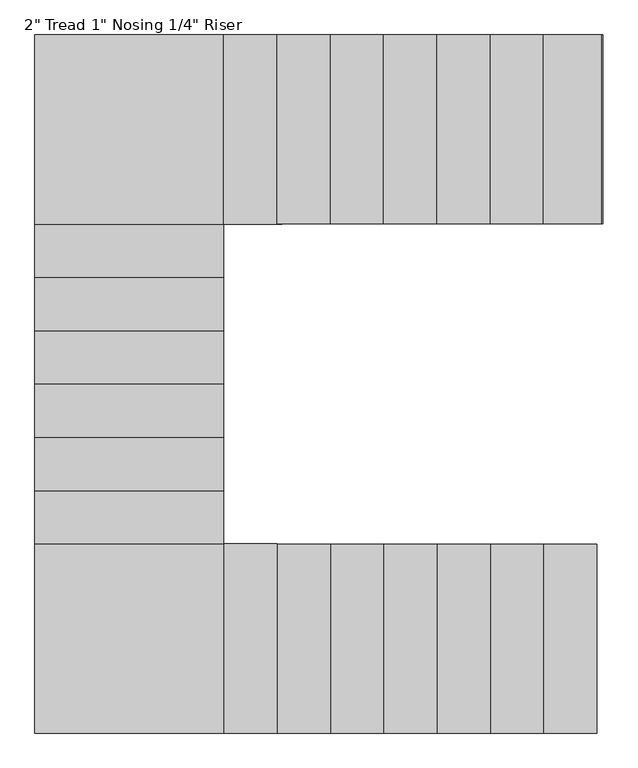
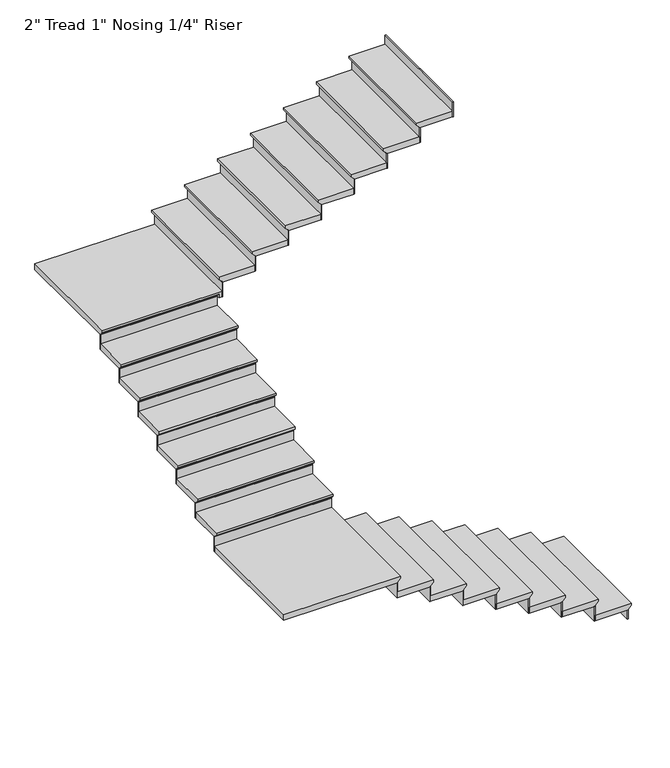
"""IFC4 building model written with IfcOpenShell, lengths in millimetres: stair flight geometry."""

from ifc_helpers import new_model, si_unit, origin, place, context, project, spatial, faceted_brep, source, transform, mapped, element, save


def stair_flight_8adf14a6(model_context):
    return source(origin(), model_context, "Body", "Brep", [
        faceted_brep([(-19769.8789184, -127.8399287, 6361.8717391), (-19769.8789184, -127.8399287, 6380.9217391), (-19769.8789184, -1118.4399287, 6380.9217391), (-19769.8789184, -1118.4399287, 6361.8717391), (-19795.2789184, -127.8399287, 6336.4717391), (-19795.2789184, -1118.4399287, 6336.4717391), (-20074.6789184, -127.8399287, 6380.9217391), (-20074.6789184, -1118.4399287, 6380.9217391), (-19795.2789184, -1118.4399287, 6330.1217391), (-20074.6789184, -1118.4399287, 6330.1217391), (-20074.6789184, -127.8399287, 6330.1217391), (-19795.2789184, -127.8399287, 6330.1217391)], [[[0, 1, 2, 3]], [[4, 0, 3, 5]], [[2, 1, 6, 7]], [[8, 9, 10, 11]], [[2, 7, 9, 8, 5, 3]], [[8, 11, 4, 5]], [[6, 1, 0, 4, 11, 10]], [[7, 6, 10, 9]]]),
        faceted_brep([(-19795.2789184, -127.8399287, 6330.1217391), (-19795.2789184, -127.8399287, 6248.4), (-19801.6289184, -127.8399287, 6248.4), (-19801.6289184, -127.8399287, 6330.1217391), (-19795.2789184, -1118.4399287, 6330.1217391), (-19801.6289184, -1118.4399287, 6330.1217391), (-19801.6289184, -1118.4399287, 6248.4), (-19795.2789184, -1118.4399287, 6248.4)], [[[0, 1, 2, 3]], [[4, 5, 6, 7]], [[1, 0, 4, 7]], [[2, 1, 7, 6]], [[3, 2, 6, 5]], [[0, 3, 5, 4]]]),
        faceted_brep([(-20074.6789184, -127.8399287, 6462.6434783), (-20074.6789184, -127.8399287, 6330.1217391), (-20081.0289184, -127.8399287, 6330.1217391), (-20081.0289184, -127.8399287, 6462.6434783), (-20074.6789184, -1118.4399287, 6462.6434783), (-20081.0289184, -1118.4399287, 6462.6434783), (-20081.0289184, -1118.4399287, 6330.1217391), (-20074.6789184, -1118.4399287, 6330.1217391)], [[[0, 1, 2, 3]], [[4, 5, 6, 7]], [[1, 0, 4, 7]], [[2, 1, 7, 6]], [[3, 2, 6, 5]], [[0, 3, 5, 4]]]),
        faceted_brep([(-20049.2789184, -1118.4399287, 6513.4434783), (-20049.2789184, -127.8399287, 6513.4434783), (-20354.0789184, -127.8399287, 6513.4434783), (-20354.0789184, -1118.4399287, 6513.4434783), (-20074.6789184, -1118.4399287, 6462.6434783), (-20354.0789184, -1118.4399287, 6462.6434783), (-20354.0789184, -127.8399287, 6462.6434783), (-20074.6789184, -127.8399287, 6462.6434783), (-20074.6789184, -1118.4399287, 6468.9934783), (-20049.2789184, -1118.4399287, 6494.3934783), (-20074.6789184, -127.8399287, 6468.9934783), (-20049.2789184, -127.8399287, 6494.3934783)], [[[0, 1, 2, 3]], [[4, 5, 6, 7]], [[0, 3, 5, 4, 8, 9]], [[4, 7, 10, 8]], [[2, 1, 11, 10, 7, 6]], [[3, 2, 6, 5]], [[11, 1, 0, 9]], [[10, 11, 9, 8]]]),
        faceted_brep([(-20354.0789184, -127.8399287, 6595.1652174), (-20354.0789184, -127.8399287, 6462.6434783), (-20360.4289184, -127.8399287, 6462.6434783), (-20360.4289184, -127.8399287, 6595.1652174), (-20354.0789184, -1118.4399287, 6595.1652174), (-20360.4289184, -1118.4399287, 6595.1652174), (-20360.4289184, -1118.4399287, 6462.6434783), (-20354.0789184, -1118.4399287, 6462.6434783)], [[[0, 1, 2, 3]], [[4, 5, 6, 7]], [[1, 0, 4, 7]], [[2, 1, 7, 6]], [[3, 2, 6, 5]], [[0, 3, 5, 4]]]),
        faceted_brep([(-20328.6789184, -1118.4399287, 6645.9652174), (-20328.6789184, -127.8399287, 6645.9652174), (-20633.4789184, -127.8399287, 6645.9652174), (-20633.4789184, -1118.4399287, 6645.9652174), (-20354.0789184, -1118.4399287, 6595.1652174), (-20633.4789184, -1118.4399287, 6595.1652174), (-20633.4789184, -127.8399287, 6595.1652174), (-20354.0789184, -127.8399287, 6595.1652174), (-20354.0789184, -1118.4399287, 6601.5152174), (-20328.6789184, -1118.4399287, 6626.9152174), (-20354.0789184, -127.8399287, 6601.5152174), (-20328.6789184, -127.8399287, 6626.9152174)], [[[0, 1, 2, 3]], [[4, 5, 6, 7]], [[0, 3, 5, 4, 8, 9]], [[4, 7, 10, 8]], [[2, 1, 11, 10, 7, 6]], [[3, 2, 6, 5]], [[11, 1, 0, 9]], [[10, 11, 9, 8]]]),
        faceted_brep([(-20633.4789184, -127.8399287, 6727.6869565), (-20633.4789184, -127.8399287, 6595.1652174), (-20639.8289184, -127.8399287, 6595.1652174), (-20639.8289184, -127.8399287, 6727.6869565), (-20633.4789184, -1118.4399287, 6727.6869565), (-20639.8289184, -1118.4399287, 6727.6869565), (-20639.8289184, -1118.4399287, 6595.1652174), (-20633.4789184, -1118.4399287, 6595.1652174)], [[[0, 1, 2, 3]], [[4, 5, 6, 7]], [[1, 0, 4, 7]], [[2, 1, 7, 6]], [[3, 2, 6, 5]], [[0, 3, 5, 4]]]),
        faceted_brep([(-20608.0789184, -1118.4399287, 6778.4869565), (-20608.0789184, -127.8399287, 6778.4869565), (-20912.8789184, -127.8399287, 6778.4869565), (-20912.8789184, -1118.4399287, 6778.4869565), (-20633.4789184, -1118.4399287, 6727.6869565), (-20912.8789184, -1118.4399287, 6727.6869565), (-20912.8789184, -127.8399287, 6727.6869565), (-20633.4789184, -127.8399287, 6727.6869565), (-20633.4789184, -1118.4399287, 6734.0369565), (-20608.0789184, -1118.4399287, 6759.4369565), (-20633.4789184, -127.8399287, 6734.0369565), (-20608.0789184, -127.8399287, 6759.4369565)], [[[0, 1, 2, 3]], [[4, 5, 6, 7]], [[0, 3, 5, 4, 8, 9]], [[4, 7, 10, 8]], [[2, 1, 11, 10, 7, 6]], [[3, 2, 6, 5]], [[11, 1, 0, 9]], [[10, 11, 9, 8]]]),
        faceted_brep([(-20912.8789184, -127.8399287, 6860.2086957), (-20912.8789184, -127.8399287, 6727.6869565), (-20919.2289184, -127.8399287, 6727.6869565), (-20919.2289184, -127.8399287, 6860.2086957), (-20912.8789184, -1118.4399287, 6860.2086957), (-20919.2289184, -1118.4399287, 6860.2086957), (-20919.2289184, -1118.4399287, 6727.6869565), (-20912.8789184, -1118.4399287, 6727.6869565)], [[[0, 1, 2, 3]], [[4, 5, 6, 7]], [[1, 0, 4, 7]], [[2, 1, 7, 6]], [[3, 2, 6, 5]], [[0, 3, 5, 4]]]),
        faceted_brep([(-20887.4789184, -1118.4399287, 6911.0086957), (-20887.4789184, -127.8399287, 6911.0086957), (-21192.2789184, -127.8399287, 6911.0086957), (-21192.2789184, -1118.4399287, 6911.0086957), (-20912.8789184, -1118.4399287, 6860.2086957), (-21192.2789184, -1118.4399287, 6860.2086957), (-21192.2789184, -127.8399287, 6860.2086957), (-20912.8789184, -127.8399287, 6860.2086957), (-20912.8789184, -1118.4399287, 6866.5586957), (-20887.4789184, -1118.4399287, 6891.9586957), (-20912.8789184, -127.8399287, 6866.5586957), (-20887.4789184, -127.8399287, 6891.9586957)], [[[0, 1, 2, 3]], [[4, 5, 6, 7]], [[0, 3, 5, 4, 8, 9]], [[4, 7, 10, 8]], [[2, 1, 11, 10, 7, 6]], [[3, 2, 6, 5]], [[11, 1, 0, 9]], [[10, 11, 9, 8]]]),
        faceted_brep([(-21192.2789184, -127.8399287, 6992.7304348), (-21192.2789184, -127.8399287, 6860.2086957), (-21198.6289184, -127.8399287, 6860.2086957), (-21198.6289184, -127.8399287, 6992.7304348), (-21192.2789184, -1118.4399287, 6992.7304348), (-21198.6289184, -1118.4399287, 6992.7304348), (-21198.6289184, -1118.4399287, 6860.2086957), (-21192.2789184, -1118.4399287, 6860.2086957)], [[[0, 1, 2, 3]], [[4, 5, 6, 7]], [[1, 0, 4, 7]], [[2, 1, 7, 6]], [[3, 2, 6, 5]], [[0, 3, 5, 4]]]),
        faceted_brep([(-21166.8789184, -1118.4399287, 7043.5304348), (-21166.8789184, -127.8399287, 7043.5304348), (-21471.6789184, -127.8399287, 7043.5304348), (-21471.6789184, -1118.4399287, 7043.5304348), (-21192.2789184, -1118.4399287, 6992.7304348), (-21471.6789184, -1118.4399287, 6992.7304348), (-21471.6789184, -127.8399287, 6992.7304348), (-21192.2789184, -127.8399287, 6992.7304348), (-21192.2789184, -1118.4399287, 6999.0804348), (-21166.8789184, -1118.4399287, 7024.4804348), (-21192.2789184, -127.8399287, 6999.0804348), (-21166.8789184, -127.8399287, 7024.4804348)], [[[0, 1, 2, 3]], [[4, 5, 6, 7]], [[0, 3, 5, 4, 8, 9]], [[4, 7, 10, 8]], [[2, 1, 11, 10, 7, 6]], [[3, 2, 6, 5]], [[11, 1, 0, 9]], [[10, 11, 9, 8]]]),
        faceted_brep([(-21471.6789184, -127.8399287, 7125.2521739), (-21471.6789184, -127.8399287, 6992.7304348), (-21478.0289184, -127.8399287, 6992.7304348), (-21478.0289184, -127.8399287, 7125.2521739), (-21471.6789184, -1118.4399287, 7125.2521739), (-21478.0289184, -1118.4399287, 7125.2521739), (-21478.0289184, -1118.4399287, 6992.7304348), (-21471.6789184, -1118.4399287, 6992.7304348)], [[[0, 1, 2, 3]], [[4, 5, 6, 7]], [[1, 0, 4, 7]], [[2, 1, 7, 6]], [[3, 2, 6, 5]], [[0, 3, 5, 4]]]),
        faceted_brep([(-21446.2789184, -1118.4399287, 7176.0521739), (-21446.2789184, -127.8399287, 7176.0521739), (-21751.0789184, -127.8399287, 7176.0521739), (-21751.0789184, -1118.4399287, 7176.0521739), (-21471.6789184, -1118.4399287, 7125.2521739), (-21751.0789184, -1118.4399287, 7125.2521739), (-21751.0789184, -127.8399287, 7125.2521739), (-21471.6789184, -127.8399287, 7125.2521739), (-21471.6789184, -1118.4399287, 7131.6021739), (-21446.2789184, -1118.4399287, 7157.0021739), (-21471.6789184, -127.8399287, 7131.6021739), (-21446.2789184, -127.8399287, 7157.0021739)], [[[0, 1, 2, 3]], [[4, 5, 6, 7]], [[0, 3, 5, 4, 8, 9]], [[4, 7, 10, 8]], [[2, 1, 11, 10, 7, 6]], [[3, 2, 6, 5]], [[11, 1, 0, 9]], [[10, 11, 9, 8]]]),
        faceted_brep([(-21751.0789184, -127.8399287, 7257.773913), (-21751.0789184, -127.8399287, 7125.2521739), (-21757.4289184, -127.8399287, 7125.2521739), (-21757.4289184, -127.8399287, 7257.773913), (-21751.0789184, -1118.4399287, 7257.773913), (-21757.4289184, -1118.4399287, 7257.773913), (-21757.4289184, -1118.4399287, 7125.2521739), (-21751.0789184, -1118.4399287, 7125.2521739)], [[[0, 1, 2, 3]], [[4, 5, 6, 7]], [[1, 0, 4, 7]], [[2, 1, 7, 6]], [[3, 2, 6, 5]], [[0, 3, 5, 4]]]),
        faceted_brep([(-22716.2789184, -102.4399287, 7308.573913), (-22716.2789184, -1118.4399287, 7308.573913), (-21725.6789184, -1118.4399287, 7308.573913), (-21725.6789184, -102.4399287, 7308.573913), (-22716.2789184, -1118.4399287, 7257.773913), (-22716.2789184, -102.4399287, 7257.773913), (-21725.6789184, -102.4399287, 7257.773913), (-21725.6789184, -127.8399287, 7257.773913), (-21751.0789184, -127.8399287, 7257.773913), (-21751.0789184, -1118.4399287, 7257.773913), (-21751.0789184, -127.8399287, 7264.123913), (-21751.0789184, -1118.4399287, 7264.123913), (-21725.6789184, -1118.4399287, 7289.523913), (-21725.6789184, -127.8399287, 7289.523913)], [[[0, 1, 2, 3]], [[4, 5, 6, 7, 8, 9]], [[1, 0, 5, 4]], [[9, 8, 10, 11]], [[3, 2, 12, 13, 7, 6]], [[0, 3, 6, 5]], [[12, 11, 10, 13]], [[2, 1, 4, 9, 11, 12]], [[8, 7, 13, 10]]]),
        faceted_brep([(-21725.6789184, -102.4399287, 7390.2956522), (-21725.6789184, -102.4399287, 7257.773913), (-21725.6789184, -96.0899287, 7257.773913), (-21725.6789184, -96.0899287, 7390.2956522), (-22716.2789184, -102.4399287, 7390.2956522), (-22716.2789184, -96.0899287, 7390.2956522), (-22716.2789184, -96.0899287, 7257.773913), (-22716.2789184, -102.4399287, 7257.773913)], [[[0, 1, 2, 3]], [[4, 5, 6, 7]], [[1, 0, 4, 7]], [[2, 1, 7, 6]], [[3, 2, 6, 5]], [[0, 3, 5, 4]]]),
        faceted_brep([(-22716.2789184, -127.8399287, 7441.0956522), (-21725.6789184, -127.8399287, 7441.0956522), (-21725.6789184, 176.9600713, 7441.0956522), (-22716.2789184, 176.9600713, 7441.0956522), (-22716.2789184, -102.4399287, 7390.2956522), (-22716.2789184, 176.9600713, 7390.2956522), (-21725.6789184, 176.9600713, 7390.2956522), (-21725.6789184, -102.4399287, 7390.2956522), (-22716.2789184, -102.4399287, 7396.6456522), (-22716.2789184, -127.8399287, 7422.0456522), (-21725.6789184, -102.4399287, 7396.6456522), (-21725.6789184, -127.8399287, 7422.0456522)], [[[0, 1, 2, 3]], [[4, 5, 6, 7]], [[0, 3, 5, 4, 8, 9]], [[4, 7, 10, 8]], [[2, 1, 11, 10, 7, 6]], [[3, 2, 6, 5]], [[11, 1, 0, 9]], [[10, 11, 9, 8]]]),
        faceted_brep([(-21725.6789184, 176.9600713, 7522.8173913), (-21725.6789184, 176.9600713, 7390.2956522), (-21725.6789184, 183.3100713, 7390.2956522), (-21725.6789184, 183.3100713, 7522.8173913), (-22716.2789184, 176.9600713, 7522.8173913), (-22716.2789184, 183.3100713, 7522.8173913), (-22716.2789184, 183.3100713, 7390.2956522), (-22716.2789184, 176.9600713, 7390.2956522)], [[[0, 1, 2, 3]], [[4, 5, 6, 7]], [[1, 0, 4, 7]], [[2, 1, 7, 6]], [[3, 2, 6, 5]], [[0, 3, 5, 4]]]),
        faceted_brep([(-22716.2789184, 151.5600713, 7573.6173913), (-21725.6789184, 151.5600713, 7573.6173913), (-21725.6789184, 456.3600713, 7573.6173913), (-22716.2789184, 456.3600713, 7573.6173913), (-22716.2789184, 176.9600713, 7522.8173913), (-22716.2789184, 456.3600713, 7522.8173913), (-21725.6789184, 456.3600713, 7522.8173913), (-21725.6789184, 176.9600713, 7522.8173913), (-22716.2789184, 176.9600713, 7529.1673913), (-22716.2789184, 151.5600713, 7554.5673913), (-21725.6789184, 176.9600713, 7529.1673913), (-21725.6789184, 151.5600713, 7554.5673913)], [[[0, 1, 2, 3]], [[4, 5, 6, 7]], [[0, 3, 5, 4, 8, 9]], [[4, 7, 10, 8]], [[2, 1, 11, 10, 7, 6]], [[3, 2, 6, 5]], [[11, 1, 0, 9]], [[10, 11, 9, 8]]]),
        faceted_brep([(-21725.6789184, 456.3600713, 7655.3391304), (-21725.6789184, 456.3600713, 7522.8173913), (-21725.6789184, 462.7100713, 7522.8173913), (-21725.6789184, 462.7100713, 7655.3391304), (-22716.2789184, 456.3600713, 7655.3391304), (-22716.2789184, 462.7100713, 7655.3391304), (-22716.2789184, 462.7100713, 7522.8173913), (-22716.2789184, 456.3600713, 7522.8173913)], [[[0, 1, 2, 3]], [[4, 5, 6, 7]], [[1, 0, 4, 7]], [[2, 1, 7, 6]], [[3, 2, 6, 5]], [[0, 3, 5, 4]]]),
        faceted_brep([(-22716.2789184, 430.9600713, 7706.1391304), (-21725.6789184, 430.9600713, 7706.1391304), (-21725.6789184, 735.7600713, 7706.1391304), (-22716.2789184, 735.7600713, 7706.1391304), (-22716.2789184, 456.3600713, 7655.3391304), (-22716.2789184, 735.7600713, 7655.3391304), (-21725.6789184, 735.7600713, 7655.3391304), (-21725.6789184, 456.3600713, 7655.3391304), (-22716.2789184, 456.3600713, 7661.6891304), (-22716.2789184, 430.9600713, 7687.0891304), (-21725.6789184, 456.3600713, 7661.6891304), (-21725.6789184, 430.9600713, 7687.0891304)], [[[0, 1, 2, 3]], [[4, 5, 6, 7]], [[0, 3, 5, 4, 8, 9]], [[4, 7, 10, 8]], [[2, 1, 11, 10, 7, 6]], [[3, 2, 6, 5]], [[11, 1, 0, 9]], [[10, 11, 9, 8]]]),
        faceted_brep([(-21725.6789184, 735.7600713, 7787.8608696), (-21725.6789184, 735.7600713, 7655.3391304), (-21725.6789184, 742.1100713, 7655.3391304), (-21725.6789184, 742.1100713, 7787.8608696), (-22716.2789184, 735.7600713, 7787.8608696), (-22716.2789184, 742.1100713, 7787.8608696), (-22716.2789184, 742.1100713, 7655.3391304), (-22716.2789184, 735.7600713, 7655.3391304)], [[[0, 1, 2, 3]], [[4, 5, 6, 7]], [[1, 0, 4, 7]], [[2, 1, 7, 6]], [[3, 2, 6, 5]], [[0, 3, 5, 4]]]),
        faceted_brep([(-22716.2789184, 710.3600713, 7838.6608696), (-21725.6789184, 710.3600713, 7838.6608696), (-21725.6789184, 1015.1600713, 7838.6608696), (-22716.2789184, 1015.1600713, 7838.6608696), (-22716.2789184, 735.7600713, 7787.8608696), (-22716.2789184, 1015.1600713, 7787.8608696), (-21725.6789184, 1015.1600713, 7787.8608696), (-21725.6789184, 735.7600713, 7787.8608696), (-22716.2789184, 735.7600713, 7794.2108696), (-22716.2789184, 710.3600713, 7819.6108696), (-21725.6789184, 735.7600713, 7794.2108696), (-21725.6789184, 710.3600713, 7819.6108696)], [[[0, 1, 2, 3]], [[4, 5, 6, 7]], [[0, 3, 5, 4, 8, 9]], [[4, 7, 10, 8]], [[2, 1, 11, 10, 7, 6]], [[3, 2, 6, 5]], [[11, 1, 0, 9]], [[10, 11, 9, 8]]]),
        faceted_brep([(-21725.6789184, 1015.1600713, 7920.3826087), (-21725.6789184, 1015.1600713, 7787.8608696), (-21725.6789184, 1021.5100713, 7787.8608696), (-21725.6789184, 1021.5100713, 7920.3826087), (-22716.2789184, 1015.1600713, 7920.3826087), (-22716.2789184, 1021.5100713, 7920.3826087), (-22716.2789184, 1021.5100713, 7787.8608696), (-22716.2789184, 1015.1600713, 7787.8608696)], [[[0, 1, 2, 3]], [[4, 5, 6, 7]], [[1, 0, 4, 7]], [[2, 1, 7, 6]], [[3, 2, 6, 5]], [[0, 3, 5, 4]]]),
        faceted_brep([(-22716.2789184, 989.7600713, 7971.1826087), (-21725.6789184, 989.7600713, 7971.1826087), (-21725.6789184, 1294.5600713, 7971.1826087), (-22716.2789184, 1294.5600713, 7971.1826087), (-22716.2789184, 1015.1600713, 7920.3826087), (-22716.2789184, 1294.5600713, 7920.3826087), (-21725.6789184, 1294.5600713, 7920.3826087), (-21725.6789184, 1015.1600713, 7920.3826087), (-22716.2789184, 1015.1600713, 7926.7326087), (-22716.2789184, 989.7600713, 7952.1326087), (-21725.6789184, 1015.1600713, 7926.7326087), (-21725.6789184, 989.7600713, 7952.1326087)], [[[0, 1, 2, 3]], [[4, 5, 6, 7]], [[0, 3, 5, 4, 8, 9]], [[4, 7, 10, 8]], [[2, 1, 11, 10, 7, 6]], [[3, 2, 6, 5]], [[11, 1, 0, 9]], [[10, 11, 9, 8]]]),
        faceted_brep([(-21725.6789184, 1294.5600713, 8052.9043478), (-21725.6789184, 1294.5600713, 7920.3826087), (-21725.6789184, 1300.9100713, 7920.3826087), (-21725.6789184, 1300.9100713, 8052.9043478), (-22716.2789184, 1294.5600713, 8052.9043478), (-22716.2789184, 1300.9100713, 8052.9043478), (-22716.2789184, 1300.9100713, 7920.3826087), (-22716.2789184, 1294.5600713, 7920.3826087)], [[[0, 1, 2, 3]], [[4, 5, 6, 7]], [[1, 0, 4, 7]], [[2, 1, 7, 6]], [[3, 2, 6, 5]], [[0, 3, 5, 4]]]),
        faceted_brep([(-22716.2789184, 1269.1600713, 8103.7043478), (-21725.6789184, 1269.1600713, 8103.7043478), (-21725.6789184, 1573.9600713, 8103.7043478), (-22716.2789184, 1573.9600713, 8103.7043478), (-22716.2789184, 1294.5600713, 8052.9043478), (-22716.2789184, 1573.9600713, 8052.9043478), (-21725.6789184, 1573.9600713, 8052.9043478), (-21725.6789184, 1294.5600713, 8052.9043478), (-22716.2789184, 1294.5600713, 8059.2543478), (-22716.2789184, 1269.1600713, 8084.6543478), (-21725.6789184, 1294.5600713, 8059.2543478), (-21725.6789184, 1269.1600713, 8084.6543478)], [[[0, 1, 2, 3]], [[4, 5, 6, 7]], [[0, 3, 5, 4, 8, 9]], [[4, 7, 10, 8]], [[2, 1, 11, 10, 7, 6]], [[3, 2, 6, 5]], [[11, 1, 0, 9]], [[10, 11, 9, 8]]]),
        faceted_brep([(-21725.6789184, 1573.9600713, 8185.426087), (-21725.6789184, 1573.9600713, 8052.9043478), (-21725.6789184, 1580.3100713, 8052.9043478), (-21725.6789184, 1580.3100713, 8185.426087), (-22716.2789184, 1573.9600713, 8185.426087), (-22716.2789184, 1580.3100713, 8185.426087), (-22716.2789184, 1580.3100713, 8052.9043478), (-22716.2789184, 1573.9600713, 8052.9043478)], [[[0, 1, 2, 3]], [[4, 5, 6, 7]], [[1, 0, 4, 7]], [[2, 1, 7, 6]], [[3, 2, 6, 5]], [[0, 3, 5, 4]]]),
        faceted_brep([(-21700.2789184, 2539.1600713, 8236.226087), (-22716.2789184, 2539.1600713, 8236.226087), (-22716.2789184, 1548.5600713, 8236.226087), (-21700.2789184, 1548.5600713, 8236.226087), (-22716.2789184, 2539.1600713, 8185.426087), (-21700.2789184, 2539.1600713, 8185.426087), (-21700.2789184, 1548.5600713, 8185.426087), (-21725.6789184, 1548.5600713, 8185.426087), (-21725.6789184, 1573.9600713, 8185.426087), (-22716.2789184, 1573.9600713, 8185.426087), (-21725.6789184, 1573.9600713, 8191.776087), (-22716.2789184, 1573.9600713, 8191.776087), (-22716.2789184, 1548.5600713, 8217.176087), (-21725.6789184, 1548.5600713, 8217.176087)], [[[0, 1, 2, 3]], [[4, 5, 6, 7, 8, 9]], [[1, 0, 5, 4]], [[9, 8, 10, 11]], [[3, 2, 12, 13, 7, 6]], [[0, 3, 6, 5]], [[12, 11, 10, 13]], [[2, 1, 4, 9, 11, 12]], [[8, 7, 13, 10]]]),
        faceted_brep([(-21700.2789184, 1548.5600713, 8317.9478261), (-21700.2789184, 1548.5600713, 8185.426087), (-21693.9289184, 1548.5600713, 8185.426087), (-21693.9289184, 1548.5600713, 8317.9478261), (-21700.2789184, 2539.1600713, 8317.9478261), (-21693.9289184, 2539.1600713, 8317.9478261), (-21693.9289184, 2539.1600713, 8185.426087), (-21700.2789184, 2539.1600713, 8185.426087)], [[[0, 1, 2, 3]], [[4, 5, 6, 7]], [[1, 0, 4, 7]], [[2, 1, 7, 6]], [[3, 2, 6, 5]], [[0, 3, 5, 4]]]),
        faceted_brep([(-21725.6789184, 2539.1600713, 8368.7478261), (-21725.6789184, 1548.5600713, 8368.7478261), (-21420.8789184, 1548.5600713, 8368.7478261), (-21420.8789184, 2539.1600713, 8368.7478261), (-21700.2789184, 2539.1600713, 8317.9478261), (-21420.8789184, 2539.1600713, 8317.9478261), (-21420.8789184, 1548.5600713, 8317.9478261), (-21700.2789184, 1548.5600713, 8317.9478261), (-21700.2789184, 2539.1600713, 8324.2978261), (-21725.6789184, 2539.1600713, 8349.6978261), (-21700.2789184, 1548.5600713, 8324.2978261), (-21725.6789184, 1548.5600713, 8349.6978261)], [[[0, 1, 2, 3]], [[4, 5, 6, 7]], [[0, 3, 5, 4, 8, 9]], [[4, 7, 10, 8]], [[2, 1, 11, 10, 7, 6]], [[3, 2, 6, 5]], [[11, 1, 0, 9]], [[10, 11, 9, 8]]]),
        faceted_brep([(-21420.8789184, 1548.5600713, 8450.4695652), (-21420.8789184, 1548.5600713, 8317.9478261), (-21414.5289184, 1548.5600713, 8317.9478261), (-21414.5289184, 1548.5600713, 8450.4695652), (-21420.8789184, 2539.1600713, 8450.4695652), (-21414.5289184, 2539.1600713, 8450.4695652), (-21414.5289184, 2539.1600713, 8317.9478261), (-21420.8789184, 2539.1600713, 8317.9478261)], [[[0, 1, 2, 3]], [[4, 5, 6, 7]], [[1, 0, 4, 7]], [[2, 1, 7, 6]], [[3, 2, 6, 5]], [[0, 3, 5, 4]]]),
        faceted_brep([(-21446.2789184, 2539.1600713, 8501.2695652), (-21446.2789184, 1548.5600713, 8501.2695652), (-21141.4789184, 1548.5600713, 8501.2695652), (-21141.4789184, 2539.1600713, 8501.2695652), (-21420.8789184, 2539.1600713, 8450.4695652), (-21141.4789184, 2539.1600713, 8450.4695652), (-21141.4789184, 1548.5600713, 8450.4695652), (-21420.8789184, 1548.5600713, 8450.4695652), (-21420.8789184, 2539.1600713, 8456.8195652), (-21446.2789184, 2539.1600713, 8482.2195652), (-21420.8789184, 1548.5600713, 8456.8195652), (-21446.2789184, 1548.5600713, 8482.2195652)], [[[0, 1, 2, 3]], [[4, 5, 6, 7]], [[0, 3, 5, 4, 8, 9]], [[4, 7, 10, 8]], [[2, 1, 11, 10, 7, 6]], [[3, 2, 6, 5]], [[11, 1, 0, 9]], [[10, 11, 9, 8]]]),
        faceted_brep([(-21141.4789184, 1548.5600713, 8582.9913043), (-21141.4789184, 1548.5600713, 8450.4695652), (-21135.1289184, 1548.5600713, 8450.4695652), (-21135.1289184, 1548.5600713, 8582.9913043), (-21141.4789184, 2539.1600713, 8582.9913043), (-21135.1289184, 2539.1600713, 8582.9913043), (-21135.1289184, 2539.1600713, 8450.4695652), (-21141.4789184, 2539.1600713, 8450.4695652)], [[[0, 1, 2, 3]], [[4, 5, 6, 7]], [[1, 0, 4, 7]], [[2, 1, 7, 6]], [[3, 2, 6, 5]], [[0, 3, 5, 4]]]),
        faceted_brep([(-21166.8789184, 2539.1600713, 8633.7913043), (-21166.8789184, 1548.5600713, 8633.7913043), (-20862.0789184, 1548.5600713, 8633.7913043), (-20862.0789184, 2539.1600713, 8633.7913043), (-21141.4789184, 2539.1600713, 8582.9913043), (-20862.0789184, 2539.1600713, 8582.9913043), (-20862.0789184, 1548.5600713, 8582.9913043), (-21141.4789184, 1548.5600713, 8582.9913043), (-21141.4789184, 2539.1600713, 8589.3413043), (-21166.8789184, 2539.1600713, 8614.7413043), (-21141.4789184, 1548.5600713, 8589.3413043), (-21166.8789184, 1548.5600713, 8614.7413043)], [[[0, 1, 2, 3]], [[4, 5, 6, 7]], [[0, 3, 5, 4, 8, 9]], [[4, 7, 10, 8]], [[2, 1, 11, 10, 7, 6]], [[3, 2, 6, 5]], [[11, 1, 0, 9]], [[10, 11, 9, 8]]]),
        faceted_brep([(-20862.0789184, 1548.5600713, 8715.5130435), (-20862.0789184, 1548.5600713, 8582.9913043), (-20855.7289184, 1548.5600713, 8582.9913043), (-20855.7289184, 1548.5600713, 8715.5130435), (-20862.0789184, 2539.1600713, 8715.5130435), (-20855.7289184, 2539.1600713, 8715.5130435), (-20855.7289184, 2539.1600713, 8582.9913043), (-20862.0789184, 2539.1600713, 8582.9913043)], [[[0, 1, 2, 3]], [[4, 5, 6, 7]], [[1, 0, 4, 7]], [[2, 1, 7, 6]], [[3, 2, 6, 5]], [[0, 3, 5, 4]]]),
        faceted_brep([(-20887.4789184, 2539.1600713, 8766.3130435), (-20887.4789184, 1548.5600713, 8766.3130435), (-20582.6789184, 1548.5600713, 8766.3130435), (-20582.6789184, 2539.1600713, 8766.3130435), (-20862.0789184, 2539.1600713, 8715.5130435), (-20582.6789184, 2539.1600713, 8715.5130435), (-20582.6789184, 1548.5600713, 8715.5130435), (-20862.0789184, 1548.5600713, 8715.5130435), (-20862.0789184, 2539.1600713, 8721.8630435), (-20887.4789184, 2539.1600713, 8747.2630435), (-20862.0789184, 1548.5600713, 8721.8630435), (-20887.4789184, 1548.5600713, 8747.2630435)], [[[0, 1, 2, 3]], [[4, 5, 6, 7]], [[0, 3, 5, 4, 8, 9]], [[4, 7, 10, 8]], [[2, 1, 11, 10, 7, 6]], [[3, 2, 6, 5]], [[11, 1, 0, 9]], [[10, 11, 9, 8]]]),
        faceted_brep([(-20582.6789184, 1548.5600713, 8848.0347826), (-20582.6789184, 1548.5600713, 8715.5130435), (-20576.3289184, 1548.5600713, 8715.5130435), (-20576.3289184, 1548.5600713, 8848.0347826), (-20582.6789184, 2539.1600713, 8848.0347826), (-20576.3289184, 2539.1600713, 8848.0347826), (-20576.3289184, 2539.1600713, 8715.5130435), (-20582.6789184, 2539.1600713, 8715.5130435)], [[[0, 1, 2, 3]], [[4, 5, 6, 7]], [[1, 0, 4, 7]], [[2, 1, 7, 6]], [[3, 2, 6, 5]], [[0, 3, 5, 4]]]),
        faceted_brep([(-20608.0789184, 2539.1600713, 8898.8347826), (-20608.0789184, 1548.5600713, 8898.8347826), (-20303.2789184, 1548.5600713, 8898.8347826), (-20303.2789184, 2539.1600713, 8898.8347826), (-20582.6789184, 2539.1600713, 8848.0347826), (-20303.2789184, 2539.1600713, 8848.0347826), (-20303.2789184, 1548.5600713, 8848.0347826), (-20582.6789184, 1548.5600713, 8848.0347826), (-20582.6789184, 2539.1600713, 8854.3847826), (-20608.0789184, 2539.1600713, 8879.7847826), (-20582.6789184, 1548.5600713, 8854.3847826), (-20608.0789184, 1548.5600713, 8879.7847826)], [[[0, 1, 2, 3]], [[4, 5, 6, 7]], [[0, 3, 5, 4, 8, 9]], [[4, 7, 10, 8]], [[2, 1, 11, 10, 7, 6]], [[3, 2, 6, 5]], [[11, 1, 0, 9]], [[10, 11, 9, 8]]]),
        faceted_brep([(-20303.2789184, 1548.5600713, 8980.5565217), (-20303.2789184, 1548.5600713, 8848.0347826), (-20296.9289184, 1548.5600713, 8848.0347826), (-20296.9289184, 1548.5600713, 8980.5565217), (-20303.2789184, 2539.1600713, 8980.5565217), (-20296.9289184, 2539.1600713, 8980.5565217), (-20296.9289184, 2539.1600713, 8848.0347826), (-20303.2789184, 2539.1600713, 8848.0347826)], [[[0, 1, 2, 3]], [[4, 5, 6, 7]], [[1, 0, 4, 7]], [[2, 1, 7, 6]], [[3, 2, 6, 5]], [[0, 3, 5, 4]]]),
        faceted_brep([(-20328.6789184, 2539.1600713, 9031.3565217), (-20328.6789184, 1548.5600713, 9031.3565217), (-20023.8789184, 1548.5600713, 9031.3565217), (-20023.8789184, 2539.1600713, 9031.3565217), (-20303.2789184, 2539.1600713, 8980.5565217), (-20023.8789184, 2539.1600713, 8980.5565217), (-20023.8789184, 1548.5600713, 8980.5565217), (-20303.2789184, 1548.5600713, 8980.5565217), (-20303.2789184, 2539.1600713, 8986.9065217), (-20328.6789184, 2539.1600713, 9012.3065217), (-20303.2789184, 1548.5600713, 8986.9065217), (-20328.6789184, 1548.5600713, 9012.3065217)], [[[0, 1, 2, 3]], [[4, 5, 6, 7]], [[0, 3, 5, 4, 8, 9]], [[4, 7, 10, 8]], [[2, 1, 11, 10, 7, 6]], [[3, 2, 6, 5]], [[11, 1, 0, 9]], [[10, 11, 9, 8]]]),
        faceted_brep([(-20023.8789184, 1548.5600713, 9113.0782609), (-20023.8789184, 1548.5600713, 8980.5565217), (-20017.5289184, 1548.5600713, 8980.5565217), (-20017.5289184, 1548.5600713, 9113.0782609), (-20023.8789184, 2539.1600713, 9113.0782609), (-20017.5289184, 2539.1600713, 9113.0782609), (-20017.5289184, 2539.1600713, 8980.5565217), (-20023.8789184, 2539.1600713, 8980.5565217)], [[[0, 1, 2, 3]], [[4, 5, 6, 7]], [[1, 0, 4, 7]], [[2, 1, 7, 6]], [[3, 2, 6, 5]], [[0, 3, 5, 4]]]),
        faceted_brep([(-19744.4789184, 1548.5600713, 9245.6), (-19744.4789184, 1548.5600713, 9113.0782609), (-19738.1289184, 1548.5600713, 9113.0782609), (-19738.1289184, 1548.5600713, 9245.6), (-19744.4789184, 2539.1600713, 9245.6), (-19738.1289184, 2539.1600713, 9245.6), (-19738.1289184, 2539.1600713, 9113.0782609), (-19744.4789184, 2539.1600713, 9113.0782609)], [[[0, 1, 2, 3]], [[4, 5, 6, 7]], [[1, 0, 4, 7]], [[2, 1, 7, 6]], [[3, 2, 6, 5]], [[0, 3, 5, 4]]]),
        faceted_brep([(-20049.2789184, 2539.1600713, 9163.8782609), (-20049.2789184, 1548.5600713, 9163.8782609), (-19744.4789184, 1548.5600713, 9163.8782609), (-19744.4789184, 2539.1600713, 9163.8782609), (-20023.8789184, 2539.1600713, 9113.0782609), (-19744.4789184, 2539.1600713, 9113.0782609), (-19744.4789184, 1548.5600713, 9113.0782609), (-20023.8789184, 1548.5600713, 9113.0782609), (-20023.8789184, 2539.1600713, 9119.4282609), (-20049.2789184, 2539.1600713, 9144.8282609), (-20023.8789184, 1548.5600713, 9119.4282609), (-20049.2789184, 1548.5600713, 9144.8282609)], [[[0, 1, 2, 3]], [[4, 5, 6, 7]], [[0, 3, 5, 4, 8, 9]], [[4, 7, 10, 8]], [[2, 1, 11, 10, 7, 6]], [[3, 2, 6, 5]], [[11, 1, 0, 9]], [[10, 11, 9, 8]]]),
    ])


if __name__ == "__main__":
    model = new_model("IFC4")
    model_context = context("Model", 3, world=origin())
    ifc_project = project(units=[si_unit("LENGTHUNIT", "METRE", prefix="MILLI")], contexts=[model_context])
    site = spatial("IfcSite", under=ifc_project)
    building = spatial("IfcBuilding", under=site)
    placement = place(None, origin())
    stair_flight_shape = stair_flight_8adf14a6(model_context)
    element("IfcStairFlight", 1, ObjectType="2\" Tread 1\" Nosing 1/4\" Riser", at=placement, inside=building, context=model_context, shape_type="MappedRepresentation", body=[
        mapped(stair_flight_shape, transform((0.0, 0.0, 0.0), x_axis=(1.0, 0.0, 0.0), y_axis=(0.0, 1.0, 0.0), z_axis=(0.0, 0.0, 1.0))),
    ])
    save(model, "model.ifc")
